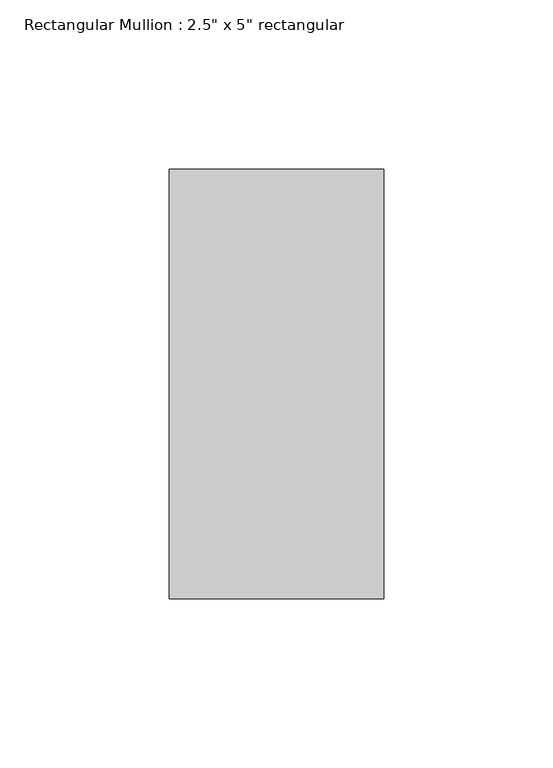
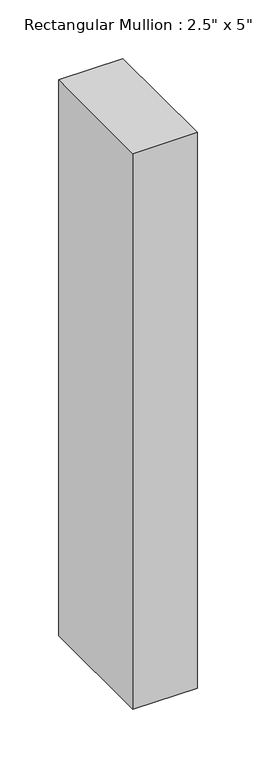
"""IFC4 building model written with IfcOpenShell, lengths in millimetres: member geometry."""

from ifc_helpers import new_model, si_unit, frame, origin, place, context, project, spatial, polyline, outline, extrude, source, transform, mapped, element, save


def member_6374d63f(model_context):
    return source(origin(), model_context, "Body", "SweptSolid", [
        extrude(outline(polyline([(31.75, 63.5), (31.75, -63.5), (-31.75, -63.5), (-31.75, 63.5), (31.75, 63.5)])), frame((0.0, 0.0, -579.9666667), z_axis=(0.0, 0.0, 1.0), x_axis=(1.0, 0.0, 0.0)), (0.0, 0.0, 1.0), 579.9666667),
    ])


if __name__ == "__main__":
    model = new_model("IFC4")
    model_context = context("Model", 3, world=origin())
    ifc_project = project(units=[si_unit("LENGTHUNIT", "METRE", prefix="MILLI")], contexts=[model_context])
    site = spatial("IfcSite", under=ifc_project)
    building = spatial("IfcBuilding", under=site)
    placement = place(None, origin())
    member_shape = member_6374d63f(model_context)
    element("IfcMember", 1, ObjectType="Rectangular Mullion : 2.5\" x 5\" rectangular", at=placement, inside=building, context=model_context, shape_type="MappedRepresentation", body=[
        mapped(member_shape, transform((0.0, 0.0, 0.0), x_axis=(1.0, 0.0, 0.0), y_axis=(0.0, 1.0, 0.0), z_axis=(0.0, 0.0, 1.0))),
    ])
    save(model, "model.ifc")

# Revit data of these elements
# Type "Rectangular Mullion : 2.5\" x 5\" rectangular"
#   built-in parameter 1007304 = 0.416667 (stored number, unit not read)
#   built-in parameter 1007301 = 0.104167 (stored number, unit not read)
#   built-in parameter 1007300 = 0.104167 (stored number, unit not read)
# Element 1 (IfcMember, "Rectangular Mullion : 2.5\" x 5\" rectangular")
#   Materials on its faces: "Aluminum"
# Materials
#   "Aluminum": class "Metal", colour RGB 247 247 247, transparency 0, Description = "Aluminum 6061", Cost = 0
